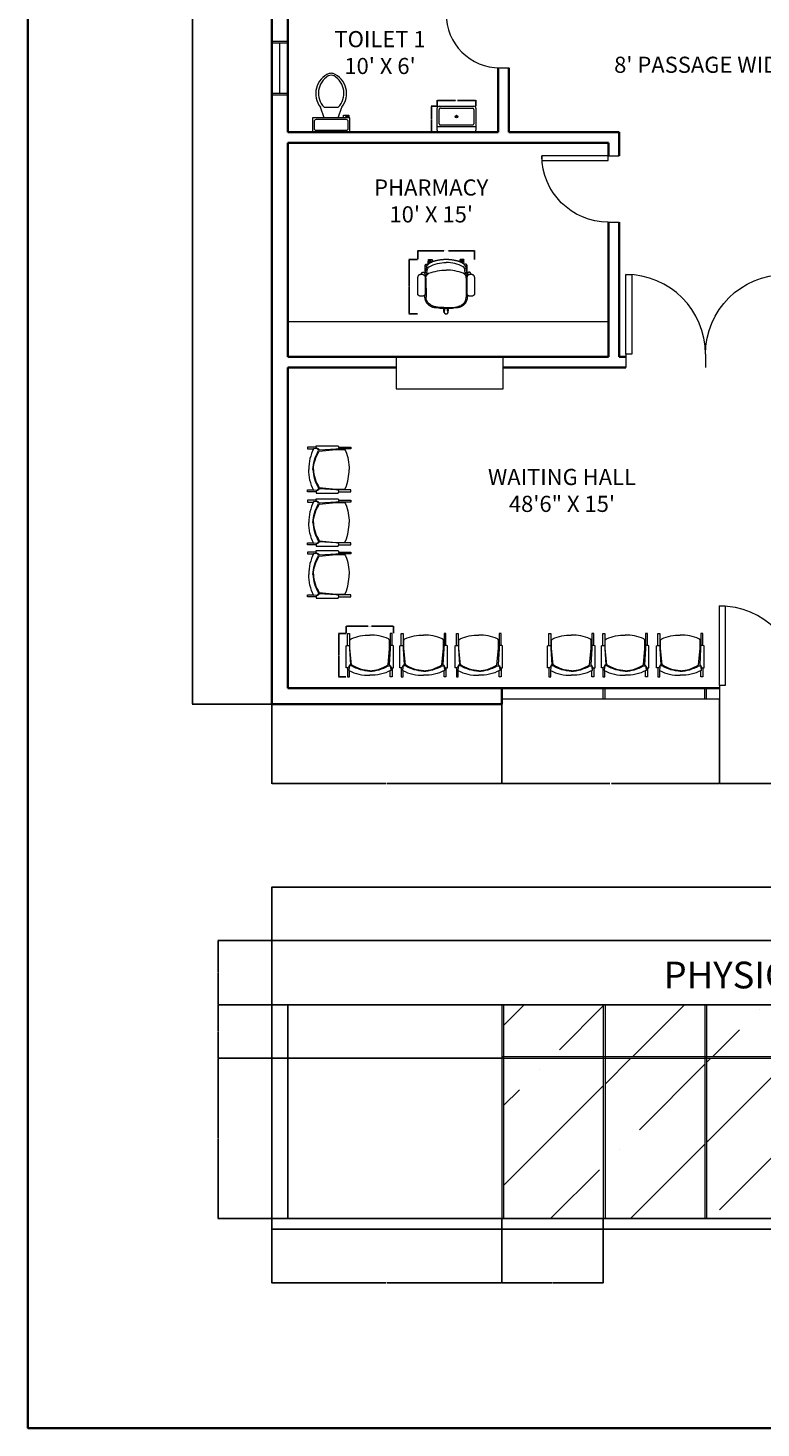
# Model space of a CAD drawing. Units: inches. Extents: x 7245 to 8143, y 15548 to 17244.
# Tile 1 of 5: x 7245 to 7657, y 15548 to 16334. Entities that reach past the tile are written whole.
import ezdxf

# ---------------------------------------------------------------- set-up
doc = ezdxf.new("R2010")
doc.units = ezdxf.units.IN
for name, color, linetype, lineweight in [('A-ANNO-DIMS', 2, 'Continuous', 18), ('A-ANNO-TEXT', 7, 'Continuous', 25), ('A-ANNO-TTLB', 7, 'Continuous', 35), ('A-AREA-IDEN', 7, 'Continuous', 18), ('A-DOOR', 3, 'Continuous', 18), ('A-ELEV', 7, 'Continuous', 25), ('A-ELEV-GLAZ', 4, 'Continuous', 18), ('A-ELEV-PATT', 252, 'Continuous', 13), ('A-FLOR-CASE', 9, 'Continuous', 20), ('A-FLOR-FIXT', 9, 'Continuous', 18), ('A-FURN', 8, 'Continuous', 18), ('A-GLAZ', 4, 'Continuous', 18), ('A-WALL', 7, 'Continuous', 35)]:
    doc.layers.add(name, color=color, linetype=linetype, lineweight=lineweight)
doc.styles.get("Standard").update_dxf_attribs({"font": 'arial.ttf'})
doc.dimstyles.get("Standard").update_dxf_attribs({"dimtxt": 0.18, "dimasz": 0.18, "dimexe": 0.18, "dimexo": 0.0625, "dimgap": 0.09, "dimtad": 0, "dimtih": 1, "dimtoh": 1, "dimdec": 4, "dimzin": 0, "dimdsep": 46, "dimtxsty": 'Standard', "dimcen": 0.09, "dimadec": 0, "dimazin": 0, "dimtfac": 1, "dimtdec": 4, "dimtofl": 0, "dimtmove": 0, "dimatfit": 3, "dimfxl": 1, "dimtolj": 1, "dimtzin": 0, "dimarcsym": 0})

# ---------------------------------------------------------------- blocks, each defined once
blk = doc.blocks.new('*U2')
for p, q in [((-600, 0), (-600, 100)), ((0, 0), (0, 100))]:
    blk.add_line(p, q)
blk.add_lwpolyline([(0, 0), (0, -600), (-43.75, -600), (-43.75, 0)], close=True)
blk.add_arc((0, 0), 600, 180, 270)
blk = doc.blocks.new('fdss')
at = {"color": 0}
for p, q in [((426, 240), (196, 239)), ((470, 236), (480, 226)), ((480, 225), (479, 223)), ((482, 204), (480, 210)), ((484, 228), (520, 224)), ((617, 196), (646, 196)), ((618, 179), (646, 179)), ((647, 195), (647, 179)), ((426, -240), (196, -239)), ((470, -236), (480, -226)), ((480, -225), (479, -223)), ((482, -204), (480, -210)), ((484, -228), (520, -224)), ((617, -196), (646, -196)), ((618, -179), (646, -179)), ((647, -195), (647, -179))]:
    blk.add_line(p, q, dxfattribs=at)
for points in [[(505, 245), (520, 247), (546, 249), (551, 249)], [(566, 236), (554, 235), (512, 240)], [(33, 21), (34, 20), (36, 19), (37, 18), (37, 18), (39, 18)], [(39, 18), (41, 17), (43, 17), (46, 16), (47, 16), (50, 16), (53, 16), (55, 16), (57, 16), (60, 16), (63, 16)], [(75, -28), (75, 0), (75, 28)], [(33, -21), (34, -20), (36, -19), (37, -18), (37, -18), (39, -18)], [(39, -18), (41, -17), (43, -17), (46, -16), (47, -16), (50, -16), (53, -16), (55, -16), (57, -16), (60, -16), (63, -16)], [(505, -245), (520, -247), (546, -249), (551, -249)], [(566, -236), (554, -235), (512, -240)]]:
    blk.add_lwpolyline(points, dxfattribs=at)
at = {"color": 0, "extrusion": (0, 0, -1)}
for centre, major_axis, start_param, end_param in [((445, 42), (-262, 262), 5.459154, 5.874691), ((201, 128), (-79, 79), 5.969012, 7.027382), ((424, 173), (47, 47), -0.751727, 0.301996), ((424, 175), (54.1, 54.1), -0.544214, -0.156468), ((514, 220), (24.9, 24.9), 3.662908, 4.015109), ((484, 224), (3.3, 3.3), 4.243712, 5.205719), ((484, 229), (-1.47, 1.47), 3.927418, 5.578652), ((-41, 3), (553, 91), -0.204201, 0.167634), ((500, 224), (-12.9, 12.9), 5.819354, 6.506047), ((509, 207), (26.9, 26.9), -1.329065, -0.883773), ((521, 177), (-33.1, 33.1), 0.763307, 1.830683), ((550, 228), (14.8, 14.8), -0.735707, 0.161366), ((545, 180), (-39.3, 39.3), 0.935679, 1.762262), ((193, 0), (-296, 296), 1.856147, 2.355859), ((566, 238), (1.31, 1.31), 0.929037, 2.293349), ((563, 238), (-2.9, 2.9), 1.793197, 2.458506), ((597, 186), (15.6, 15.6), -0.947253, 1.474381), ((621, 198), (-1.12, 1.12), 2.396655, 3.926991), ((621, 177), (-1.12, 1.12), 0.785398, 2.315734), ((646, 195), (0.539, 0.539), -0.785398, 0.785398), ((646, 179), (-0.539, 0.539), 2.356195, 3.926991)]:
    blk.add_ellipse(centre, major_axis=major_axis, ratio=1, start_param=start_param, end_param=end_param, dxfattribs=at)
at = {"color": 0}
for centre, major_axis, start_param, end_param in [((445, -42), (262, 262), 2.317561, 2.733098), ((-41, -3), (-553, 91), 2.937392, 3.309227), ((193, 0), (296, 296), 4.99774, 5.497452), ((201, -128), (79, 79), 2.82742, 3.885789), ((424, -173), (-47, 47), 2.389866, 3.443588), ((424, -175), (-54.1, 54.1), 2.597378, 2.985125), ((514, -220), (-24.9, 24.9), 0.521315, 0.873517), ((484, -224), (-3.3, 3.3), 1.102119, 2.064126), ((484, -229), (1.47, 1.47), 0.785825, 2.437059), ((500, -224), (12.9, 12.9), 2.677762, 3.364454), ((509, -207), (-26.9, 26.9), 1.812527, 2.25782), ((521, -177), (33.1, 33.1), 3.9049, 4.972275), ((550, -228), (-14.8, 14.8), 2.405886, 3.302959), ((545, -180), (39.3, 39.3), 4.077272, 4.903855), ((566, -238), (-1.31, 1.31), 4.07063, 5.434941), ((563, -238), (2.9, 2.9), 4.93479, 5.600098), ((597, -186), (15.6, 15.6), 3.765136, 6.18677), ((621, -177), (1.12, 1.12), 3.926991, 5.457327), ((621, -198), (1.12, 1.12), 5.538248, 7.068583), ((646, -179), (0.539, 0.539), 5.497787, 7.068583), ((646, -195), (-0.539, 0.539), 2.356195, 3.926991)]:
    blk.add_ellipse(centre, major_axis=major_axis, ratio=1, start_param=start_param, end_param=end_param, dxfattribs=at)
for points, weights, knots in [([(436, 337), (338, 337), (240, 337), (234, 338), (228, 335), (217, 328), (212, 315), (204, 293), (212, 271), (217, 258), (228, 251), (234, 248), (240, 248)], [1, 1, 1, 0.962754439438, 1, 0.939418827348, 1, 0.934055427035, 1, 0.939418827348, 1, 0.962754439438, 1], [0, 0, 0, 1, 1, 1.54757, 1.54757, 2.247301, 2.247301, 2.977684, 2.977684, 3.677415, 3.677415, 4.224984, 4.224984, 4.224984]), ([(436, 337), (443, 338), (449, 335), (460, 328), (464, 315), (473, 293), (464, 271), (460, 258), (449, 251), (443, 248), (436, 248), (338, 248), (240, 248)], [1, 0.96275443944, 1, 0.939418827348, 1, 0.934055427035, 1, 0.939418827348, 1, 0.96275443944, 1, 1, 1], [0, 0, 0, 0.54757, 0.54757, 1.247301, 1.247301, 1.977684, 1.977684, 2.677415, 2.677415, 3.224984, 3.224984, 4.224984, 4.224984, 4.224984]), ([(227, 252), (219, 252), (211, 252), (156, 255), (115, 218), (74, 180), (72, 125), (63, 75), (63, 25), (63, 13), (62, 0), (63, -13), (63, -25), (63, -75), (72, -125), (74, -180), (115, -218), (156, -255), (211, -252), (219, -252), (227, -252)], [1, 1, 1, 0.920970329426, 1, 0.920970329426, 1, 0.996764637726, 1, 1, 1, 1, 1, 0.996764637726, 1, 0.920970329426, 1, 0.920970329426, 1, 1, 1], [0, 0, 0, 1, 1, 1.800466, 1.800466, 2.600931, 2.600931, 2.761856, 2.761856, 3.761856, 3.761856, 4.761856, 4.761856, 4.922781, 4.922781, 5.723247, 5.723247, 6.523712, 6.523712, 7.523712, 7.523712, 7.523712]), ([(447, 248), (506, 249), (566, 251), (577, 251), (585, 244), (591, 239), (592, 232), (592, 228), (590, 225), (589, 221), (585, 219)], [1, 1, 1, 0.935512434708, 1, 0.918468104225, 1, 0.965843473499, 1, 0.972653000165, 1], [0, 0, 0, 1, 1, 1.722179, 1.722179, 2.535393, 2.535393, 3.059628, 3.059628, 3.528435, 3.528435, 3.528435]), ([(468, 296), (480, 296), (489, 288), (493, 285), (494, 280), (496, 274), (494, 268), (488, 255), (474, 254), (463, 254), (452, 253)], [1, 0.943338632687, 1, 0.968267368414, 1, 0.9394851057, 1, 0.864198855487, 1, 1, 1], [0, 0, 0, 0.676489, 0.676489, 1.181677, 1.181677, 1.881021, 1.881021, 2.935502, 2.935502, 3.935502, 3.935502, 3.935502]), ([(591, 211), (619, 173), (629, 128), (645, 65), (645, 0), (645, -65), (629, -128), (619, -173), (591, -211)], [1, 0.979760898136, 1, 0.992391068779, 1, 0.992391068779, 1, 0.979760898136, 1], [0, 0, 0, 0.403066, 0.403066, 0.649944, 0.649944, 0.896822, 0.896822, 1.299888, 1.299888, 1.299888]), ([(592, 211), (618, 216), (643, 209), (646, 209), (646, 206), (646, 203), (646, 199), (646, 198), (644, 198), (630, 198), (616, 198)], [1, 0.974666881773, 1, 0.783317345499, 1, 1, 1, 0.707106807826, 1, 1, 1], [0, 0, 0, 0.451139, 0.451139, 1.792762, 1.792762, 2.792762, 2.792762, 4.363559, 4.363559, 5.363559, 5.363559, 5.363559]), ([(618, 177), (631, 177), (644, 177), (645, 177), (645, 176), (646, 176), (646, 175), (646, 172), (646, 168), (646, 166), (643, 165), (631, 161), (619, 161)], [1, 1, 1, 0.923879528314, 1, 0.923879528314, 1, 1, 1, 0.783317456604, 1, 0.992237440768, 1], [0, 0, 0, 1, 1, 1.785398, 1.785398, 2.570796, 2.570796, 3.570796, 3.570796, 4.912419, 4.912419, 5.161781, 5.161781, 5.161781]), ([(33, -20), (22, -27), (10, -20), (-1, -13), (0, 0), (-1, 13), (10, 20), (22, 27), (33, 20)], [1, 0.85579821339, 1, 0.85579821339, 1, 0.855798213391, 1, 0.855798213391, 1], [0, 0, 0, 1.087409, 1.087409, 2.174818, 2.174818, 3.262227, 3.262227, 4.349636, 4.349636, 4.349636]), ([(12, 21), (13, 23), (15, 23), (39, 29), (63, 25)], [1, 0.873023611703, 1, 0.980536821249, 1], [0, 0, 0, 1.018856, 1.018856, 1.414094, 1.414094, 1.414094]), ([(12, -21), (13, -23), (15, -23), (39, -29), (63, -25)], [1, 0.873023611717, 1, 0.980536821249, 1], [0, 0, 0, 1.018856, 1.018856, 1.414094, 1.414094, 1.414094]), ([(618, -177), (631, -177), (644, -177), (645, -177), (645, -176), (646, -176), (646, -175), (646, -172), (646, -168), (646, -166), (643, -165), (631, -161), (619, -161)], [1, 1, 1, 0.923879528318, 1, 0.923879528318, 1, 1, 1, 0.783317456602, 1, 0.992237440768, 1], [0, 0, 0, 1, 1, 1.785398, 1.785398, 2.570796, 2.570796, 3.570796, 3.570796, 4.912419, 4.912419, 5.161781, 5.161781, 5.161781]), ([(464, -271), (460, -258), (449, -251), (443, -248), (436, -248), (338, -248), (240, -248), (234, -248), (228, -251), (217, -258), (212, -271), (204, -293), (212, -315), (217, -328), (228, -335), (234, -338), (240, -337), (338, -337), (436, -337)], [1, 0.939418827349, 1, 0.96275443944, 1, 1, 1, 0.962754439438, 1, 0.939418827349, 1, 0.934055427035, 1, 0.939418827348, 1, 0.962754439438, 1, 1, 1], [0, 0, 0, 0.699731, 0.699731, 1.247301, 1.247301, 2.247301, 2.247301, 2.794871, 2.794871, 3.494602, 3.494602, 4.224984, 4.224984, 4.924715, 4.924715, 5.472285, 5.472285, 6.472285, 6.472285, 6.472285]), ([(464, -271), (473, -293), (464, -315), (460, -328), (449, -335), (443, -338), (436, -337)], [1, 0.934055427035, 1, 0.939418827348, 1, 0.96275443944, 1], [0, 0, 0, 0.730383, 0.730383, 1.430114, 1.430114, 1.977684, 1.977684, 1.977684]), ([(447, -248), (506, -249), (566, -251), (577, -251), (585, -244), (591, -239), (592, -232), (592, -228), (590, -225), (589, -221), (585, -219)], [1, 1, 1, 0.935512434708, 1, 0.918468104224, 1, 0.965843473499, 1, 0.972653000166, 1], [0, 0, 0, 1, 1, 1.722179, 1.722179, 2.535393, 2.535393, 3.059628, 3.059628, 3.528435, 3.528435, 3.528435]), ([(468, -296), (480, -296), (489, -288), (493, -285), (494, -280), (496, -274), (494, -268), (488, -255), (474, -254), (463, -254), (452, -253)], [1, 0.943338632687, 1, 0.968267368413, 1, 0.9394851057, 1, 0.864198855486, 1, 1, 1], [0, 0, 0, 0.676489, 0.676489, 1.181677, 1.181677, 1.881021, 1.881021, 2.935502, 2.935502, 3.935502, 3.935502, 3.935502]), ([(592, -211), (618, -216), (643, -209), (646, -209), (646, -206), (646, -203), (646, -199), (646, -198), (644, -198), (630, -198), (616, -198)], [1, 0.974666881774, 1, 0.7833173455, 1, 1, 1, 0.707106807832, 1, 1, 1], [0, 0, 0, 0.451139, 0.451139, 1.792762, 1.792762, 2.792762, 2.792762, 4.363559, 4.363559, 5.363559, 5.363559, 5.363559])]:
    blk.add_rational_spline(points, weights, degree=2, knots=knots, dxfattribs=at)
blk = doc.blocks.new('chair033')
at = {"color": 0, "lineweight": -2}
for points in [[(-230, -108), (-230, 17), (-210, 17), (-210, -113)], [(230, -108), (230, 17), (210, 17), (210, -113)], [(-230, -338), (-230, -428), (-210, -428), (-210, -366)], [(230, -338), (230, -428), (210, -428), (210, -366)]]:
    blk.add_lwpolyline(points, dxfattribs=at)
for points in [[(1, -367, -0.129806), (-187, -307), (-204, -137), (-204, -56, -0.30894), (-191, -37, -0.09648), (0, 0, -0.09648)], [(-1, -367, 0.129806), (187, -307), (204, -137), (204, -56, 0.30894), (191, -37, 0.09648), (0, 0, 0.09648)], [(1, -372, -0.119401), (-187, -317, 0.398658), (-212, -327), (-215, -363, 0.13244), (0, -413)], [(-1, -372, 0.119401), (187, -317, -0.398658), (212, -327), (215, -363, -0.13244), (0, -413)]]:
    blk.add_lwpolyline(points, format="xyb", dxfattribs=at)
for points in [[(-244, -337), (-244, -157), (-244, -112, -0.285714), (-209, -112), (-209, -137), (-199, -306, 0.220172), (-212, -317), (-222, -337)], [(244, -337), (244, -157), (244, -112, 0.285714), (209, -112), (209, -137), (199, -306, -0.220172), (212, -317), (222, -337)]]:
    blk.add_lwpolyline(points, format="xyb", close=True, dxfattribs=at)
blk = doc.blocks.new('*U9')
for p, q in [((0, 0), (0, 100)), ((600, 0), (600, 100))]:
    blk.add_line(p, q)
blk.add_lwpolyline([(0, 0), (0, -600), (43.75, -600), (43.75, 0)], close=True)
blk.add_arc((0, 0), 600, 270, 0)
blk = doc.blocks.new('Toilet - top')
for p, q in [((9.5, -6), (9.5, -2)), ((-10, -8.5), (-8, -8.5)), ((-10, -9.5), (-10, -8.5)), ((-7, -9.5), (-10, -9.5)), ((-8, -8.5), (-8, -8)), ((-7, -8), (-7, -9.5)), ((-4, -8), (-6, -14)), ((4, -14), (-4, -14)), ((4, -8), (6, -14))]:
    blk.add_line(p, q)
blk.add_lwpolyline([(10.5, -8), (10.5, 0), (-10.5, 0), (-10.5, -8)], close=True)
for points in [[(-9.5, -2), (-9.5, -6)], [(8.5, -1), (-8.5, -1)], [(-8.5, -7), (8.5, -7)]]:
    blk.add_lwpolyline(points)
for centre, radius, start, end in [((-8.62, -1.88), 0.884, 81.8699, 188.1301), ((-8.62, -6.12), 0.884, 171.8699, 278.1301), ((8.62, -1.88), 0.884, 351.8699, 98.1301), ((8.62, -6.12), 0.884, 261.8699, 8.1301), ((3.52, -21.58), 12.17, 141.46911, 247.97143), ((4.2, -21.82), 11.33, 136.36773, 238.94682), ((-3.52, -21.58), 12.17, 292.02843, 38.53071), ((-4.2, -21.82), 11.33, 301.05301, 43.63209), ((0, -27.88), 4, 245.73182, 294.26817), ((0, -29), 4, 254.86053, 285.13947)]:
    blk.add_arc(centre, radius, start, end)
blk = doc.blocks.new('Sink-single - 30 in top')
blk.add_line((-15, -3.999996), (15, -3.999996))
for points in [[(-13.5, 0), (13.5, 0)], [(-15, -18.499996), (-15, -1.5)], [(-13.5, -17.499996), (-13.5, -6.499996)], [(-12.5, -5.499996), (12.5, -5.499996)], [(13.5, -6.499996), (13.5, -17.499996)], [(15, -1.5), (15, -18.499996)], [(13.5, -19.999996), (-13.5, -19.999996)], [(12.5, -18.499996), (-12.5, -18.499996)]]:
    blk.add_lwpolyline(points)
for radius in [1, 0.5]:
    blk.add_circle((0, -11.999996), radius)
for centre, radius, start, end in [((-13.5, -1.5), 1.5, 90, 180), ((-12.5, -6.499996), 1, 90, 180), ((12.5, -6.499996), 1, 0, 90), ((13.5, -1.5), 1.5, 0, 90), ((-13.5, -18.499996), 1.5, 180, 270), ((-12.5, -17.499996), 1, 180, 270), ((12.5, -17.499996), 1, 270, 0), ((13.5, -18.499996), 1.5, 270, 0)]:
    blk.add_arc(centre, radius, start, end)
blk = doc.blocks.new('WINDOW-30IN-PLAN')
for p, q in [((30, 9), (0, 9)), ((0, 9), (0, 0)), ((1, 9), (1, 0)), ((29, 0), (29, 9)), ((30, 0), (30, 9)), ((29, 4.5), (1, 4.5)), ((0, 0), (30, 0))]:
    blk.add_line(p, q)
blk = doc.blocks.new('*D18')
at = {"layer": 'A-ANNO-DIMS', "color": 0, "lineweight": -2, "transparency": 16777216}
for p, q in [((7423.74, 15993.99), (7423.74, 15998.1)), ((7423.92, 15997.92), (7436.12, 15997.92)), ((7450.22, 15997.92), (7438.02, 15997.92)), ((7450.4, 15993.99), (7450.4, 15998.1))]:
    blk.add_line(p, q, dxfattribs=at)
at = {"layer": 'A-ANNO-DIMS', "color": 0, "transparency": 16777216}
for points in [[(7423.92, 15997.95), (7423.92, 15997.89), (7423.74, 15997.92)], [(7450.22, 15997.95), (7450.22, 15997.89), (7450.4, 15997.92)]]:
    blk.add_solid(points, dxfattribs=at)
at = {"layer": 'Defpoints', "color": 0, "transparency": 16777216}
for p in [(7423.74, 15993.93), (7450.4, 15997.92), (7450.4, 15993.93)]:
    blk.add_point(p, dxfattribs=at)
at = {"layer": 'A-ANNO-DIMS', "color": 0, "transparency": 16777216, "insert": (7437.07, 15997.92), "char_height": 0.18, "attachment_point": 5}
blk.add_mtext('\\A1;CHAIR 27 TYP.', dxfattribs=at)
blk = doc.blocks.new('*D19')
at = {"layer": 'A-ANNO-DIMS', "color": 0, "lineweight": -2, "transparency": 16777216}
for p, q in [((7423.68, 15993.93), (7419.56, 15993.93)), ((7419.74, 15993.75), (7419.74, 15981.95)), ((7419.74, 15969.79), (7419.74, 15981.59)), ((7423.68, 15969.61), (7419.56, 15969.61))]:
    blk.add_line(p, q, dxfattribs=at)
at = {"layer": 'A-ANNO-DIMS', "color": 0, "transparency": 16777216}
for points in [[(7419.71, 15993.75), (7419.77, 15993.75), (7419.74, 15993.93)], [(7419.71, 15969.79), (7419.77, 15969.79), (7419.74, 15969.61)]]:
    blk.add_solid(points, dxfattribs=at)
at = {"layer": 'Defpoints', "color": 0, "transparency": 16777216}
for p in [(7419.74, 15993.93), (7423.74, 15993.93), (7423.74, 15969.61)]:
    blk.add_point(p, dxfattribs=at)
at = {"layer": 'A-ANNO-DIMS', "color": 0, "transparency": 16777216, "insert": (7419.74, 15981.77), "char_height": 0.18, "attachment_point": 5}
blk.add_mtext('\\A1;24 TYP.', dxfattribs=at)
blk = doc.blocks.new('*D24')
at = {"layer": 'A-ANNO-DIMS', "color": 0, "lineweight": -2, "transparency": 16777216}
for p, q in [((7474.87, 16289.75), (7474.87, 16293.13)), ((7475.05, 16292.95), (7485.12, 16292.95)), ((7496.43, 16292.95), (7486.37, 16292.95)), ((7496.61, 16289.75), (7496.61, 16293.13))]:
    blk.add_line(p, q, dxfattribs=at)
at = {"layer": 'A-ANNO-DIMS', "color": 0, "transparency": 16777216}
for points in [[(7475.05, 16292.98), (7475.05, 16292.92), (7474.87, 16292.95)], [(7496.43, 16292.98), (7496.43, 16292.92), (7496.61, 16292.95)]]:
    blk.add_solid(points, dxfattribs=at)
at = {"layer": 'Defpoints', "color": 0, "transparency": 16777216}
for p in [(7474.87, 16292.95), (7474.87, 16289.69), (7496.61, 16289.69)]:
    blk.add_point(p, dxfattribs=at)
at = {"layer": 'A-ANNO-DIMS', "color": 0, "transparency": 16777216, "insert": (7485.74, 16292.95), "char_height": 0.18, "attachment_point": 5}
blk.add_mtext('\\A1;BASIN 22', dxfattribs=at)
blk = doc.blocks.new('*D25')
at = {"layer": 'A-ANNO-DIMS', "color": 0, "lineweight": -2, "transparency": 16777216}
for p, q in [((7474.81, 16289.69), (7471.43, 16289.69)), ((7471.61, 16289.51), (7471.61, 16282.62)), ((7474.81, 16275.19), (7471.43, 16275.19)), ((7471.61, 16275.37), (7471.61, 16282.26))]:
    blk.add_line(p, q, dxfattribs=at)
at = {"layer": 'A-ANNO-DIMS', "color": 0, "transparency": 16777216}
for points in [[(7471.58, 16289.51), (7471.64, 16289.51), (7471.61, 16289.69)], [(7471.58, 16275.37), (7471.64, 16275.37), (7471.61, 16275.19)]]:
    blk.add_solid(points, dxfattribs=at)
at = {"layer": 'Defpoints', "color": 0, "transparency": 16777216}
for p in [(7474.87, 16289.69), (7471.61, 16275.19), (7474.87, 16275.19)]:
    blk.add_point(p, dxfattribs=at)
at = {"layer": 'A-ANNO-DIMS', "color": 0, "transparency": 16777216, "insert": (7471.61, 16282.44), "char_height": 0.18, "attachment_point": 5}
blk.add_mtext('\\A1;14', dxfattribs=at)
blk = doc.blocks.new('*D26')
at = {"layer": 'A-ANNO-DIMS', "color": 0, "lineweight": -2, "transparency": 16777216}
for p, q in [((7463.99, 16203.82), (7463.99, 16208.71)), ((7464.17, 16208.53), (7478.58, 16208.53)), ((7495.64, 16208.53), (7481.23, 16208.53)), ((7495.82, 16203.81), (7495.82, 16208.71))]:
    blk.add_line(p, q, dxfattribs=at)
at = {"layer": 'A-ANNO-DIMS', "color": 0, "transparency": 16777216}
for points in [[(7464.17, 16208.56), (7464.17, 16208.5), (7463.99, 16208.53)], [(7495.64, 16208.56), (7495.64, 16208.5), (7495.82, 16208.53)]]:
    blk.add_solid(points, dxfattribs=at)
at = {"layer": 'Defpoints', "color": 0, "transparency": 16777216}
for p in [(7495.82, 16208.53), (7463.99, 16203.75), (7495.82, 16203.75)]:
    blk.add_point(p, dxfattribs=at)
at = {"layer": 'A-ANNO-DIMS', "color": 0, "transparency": 16777216, "insert": (7479.91, 16208.53), "char_height": 0.18, "attachment_point": 5}
blk.add_mtext('\\A1;DESK CHAIR 32 TYP.', dxfattribs=at)
blk = doc.blocks.new('*D27')
at = {"layer": 'A-ANNO-DIMS', "color": 0, "lineweight": -2, "transparency": 16777216}
for p, q in [((7463.93, 16203.75), (7459.03, 16203.75)), ((7459.21, 16203.57), (7459.21, 16188.68)), ((7459.21, 16173.42), (7459.21, 16188.31)), ((7463.92, 16173.24), (7459.03, 16173.24))]:
    blk.add_line(p, q, dxfattribs=at)
at = {"layer": 'A-ANNO-DIMS', "color": 0, "transparency": 16777216}
for points in [[(7459.18, 16203.57), (7459.24, 16203.57), (7459.21, 16203.75)], [(7459.18, 16173.42), (7459.24, 16173.42), (7459.21, 16173.24)]]:
    blk.add_solid(points, dxfattribs=at)
at = {"layer": 'Defpoints', "color": 0, "transparency": 16777216}
for p in [(7459.21, 16203.75), (7463.99, 16203.75), (7463.99, 16173.24)]:
    blk.add_point(p, dxfattribs=at)
at = {"layer": 'A-ANNO-DIMS', "color": 0, "transparency": 16777216, "insert": (7459.21, 16188.5), "char_height": 0.18, "attachment_point": 5}
blk.add_mtext('\\A1;31 TYP.', dxfattribs=at)
blk = doc.blocks.new('*D43')
at = {"layer": 'A-ANNO-DIMS', "color": 0, "lineweight": -2, "transparency": 16777216}
for p, q in [((7382.02, 16842.19), (7337.4, 16842.19)), ((7337.58, 16842.01), (7337.58, 16398.37)), ((7337.58, 15954.37), (7337.58, 16398.01)), ((7382.02, 15954.19), (7337.4, 15954.19))]:
    blk.add_line(p, q, dxfattribs=at)
at = {"layer": 'A-ANNO-DIMS', "color": 0, "transparency": 16777216}
for points in [[(7337.55, 16842.01), (7337.61, 16842.01), (7337.58, 16842.19)], [(7337.55, 15954.37), (7337.61, 15954.37), (7337.58, 15954.19)]]:
    blk.add_solid(points, dxfattribs=at)
at = {"layer": 'Defpoints', "color": 0, "transparency": 16777216}
for p in [(7337.58, 16842.19), (7382.08, 16842.19), (7382.08, 15954.19)]:
    blk.add_point(p, dxfattribs=at)
at = {"layer": 'A-ANNO-DIMS', "color": 0, "transparency": 16777216, "insert": (7337.58, 16398.19), "char_height": 0.18, "attachment_point": 5}
blk.add_mtext('\\A1;888', dxfattribs=at)
blk = doc.blocks.new('*D44')
at = {"layer": 'A-ANNO-DIMS', "color": 0, "lineweight": -2, "transparency": 16777216}
for p, q in [((7382.08, 15954.13), (7382.08, 15909.51)), ((7511.08, 15954.13), (7511.08, 15909.51)), ((7382.26, 15909.69), (7446.3, 15909.69)), ((7510.9, 15909.69), (7446.86, 15909.69))]:
    blk.add_line(p, q, dxfattribs=at)
at = {"layer": 'A-ANNO-DIMS', "color": 0, "transparency": 16777216}
for points in [[(7382.26, 15909.72), (7382.26, 15909.66), (7382.08, 15909.69)], [(7510.9, 15909.72), (7510.9, 15909.66), (7511.08, 15909.69)]]:
    blk.add_solid(points, dxfattribs=at)
at = {"layer": 'Defpoints', "color": 0, "transparency": 16777216}
for p in [(7382.08, 15954.19), (7511.08, 15954.19), (7511.08, 15909.69)]:
    blk.add_point(p, dxfattribs=at)
at = {"layer": 'A-ANNO-DIMS', "color": 0, "transparency": 16777216, "insert": (7446.58, 15909.69), "char_height": 0.18, "attachment_point": 5}
blk.add_mtext('\\A1;129', dxfattribs=at)
blk = doc.blocks.new('*D45')
at = {"layer": 'A-ANNO-DIMS', "color": 0, "lineweight": -2, "transparency": 16777216}
for p, q in [((7511.08, 15957.13), (7511.08, 15909.51)), ((7633.26, 15957.13), (7633.26, 15909.51)), ((7511.26, 15909.69), (7571.72, 15909.69)), ((7633.08, 15909.69), (7572.63, 15909.69))]:
    blk.add_line(p, q, dxfattribs=at)
at = {"layer": 'A-ANNO-DIMS', "color": 0, "transparency": 16777216}
for points in [[(7511.26, 15909.72), (7511.26, 15909.66), (7511.08, 15909.69)], [(7633.08, 15909.72), (7633.08, 15909.66), (7633.26, 15909.69)]]:
    blk.add_solid(points, dxfattribs=at)
at = {"layer": 'Defpoints', "color": 0, "transparency": 16777216}
for p in [(7511.08, 15957.19), (7633.26, 15957.19), (7633.26, 15909.69)]:
    blk.add_point(p, dxfattribs=at)
at = {"layer": 'A-ANNO-DIMS', "color": 0, "transparency": 16777216, "insert": (7572.17, 15909.69), "char_height": 0.18, "attachment_point": 5}
blk.add_mtext('\\A1;122.18', dxfattribs=at)
blk = doc.blocks.new('*D46')
at = {"layer": 'A-ANNO-DIMS', "color": 0, "lineweight": -2, "transparency": 16777216}
for p, q in [((7633.26, 15957.13), (7633.26, 15909.51)), ((7722.64, 15957.13), (7722.64, 15909.51)), ((7633.44, 15909.69), (7677.55, 15909.69)), ((7722.46, 15909.69), (7678.34, 15909.69))]:
    blk.add_line(p, q, dxfattribs=at)
at = {"layer": 'A-ANNO-DIMS', "color": 0, "transparency": 16777216}
for points in [[(7633.44, 15909.72), (7633.44, 15909.66), (7633.26, 15909.69)], [(7722.46, 15909.72), (7722.46, 15909.66), (7722.64, 15909.69)]]:
    blk.add_solid(points, dxfattribs=at)
at = {"layer": 'Defpoints', "color": 0, "transparency": 16777216}
for p in [(7633.26, 15957.19), (7722.64, 15957.19), (7722.64, 15909.69)]:
    blk.add_point(p, dxfattribs=at)
at = {"layer": 'A-ANNO-DIMS', "color": 0, "transparency": 16777216, "insert": (7677.95, 15909.69), "char_height": 0.18, "attachment_point": 5}
blk.add_mtext('\\A1;89.37', dxfattribs=at)
blk = doc.blocks.new('*D69')
at = {"layer": 'A-ANNO-DIMS', "color": 0, "lineweight": -2, "transparency": 16777216}
for p, q in [((7382.08, 15821.68), (7382.08, 15851.81)), ((7382.26, 15851.63), (7681.79, 15851.63)), ((7981.9, 15851.63), (7682.37, 15851.63)), ((7982.08, 15821.68), (7982.08, 15851.81))]:
    blk.add_line(p, q, dxfattribs=at)
at = {"layer": 'A-ANNO-DIMS', "color": 0, "transparency": 16777216}
for points in [[(7382.26, 15851.66), (7382.26, 15851.6), (7382.08, 15851.63)], [(7981.9, 15851.66), (7981.9, 15851.6), (7982.08, 15851.63)]]:
    blk.add_solid(points, dxfattribs=at)
at = {"layer": 'Defpoints', "color": 0, "transparency": 16777216}
for p in [(7982.08, 15851.63), (7382.08, 15821.62), (7982.08, 15821.62)]:
    blk.add_point(p, dxfattribs=at)
at = {"layer": 'A-ANNO-DIMS', "color": 0, "transparency": 16777216, "insert": (7682.08, 15851.63), "char_height": 0.18, "attachment_point": 5}
blk.add_mtext('\\A1;600', dxfattribs=at)
blk = doc.blocks.new('*D71')
at = {"layer": 'A-ANNO-DIMS', "color": 0, "lineweight": -2, "transparency": 16777216}
for p, q in [((7382.08, 15665.56), (7382.08, 15629.42)), ((7511.08, 15665.56), (7511.08, 15629.42)), ((7382.26, 15629.6), (7446.3, 15629.6)), ((7510.9, 15629.6), (7446.86, 15629.6))]:
    blk.add_line(p, q, dxfattribs=at)
at = {"layer": 'A-ANNO-DIMS', "color": 0, "transparency": 16777216}
for points in [[(7382.26, 15629.63), (7382.26, 15629.57), (7382.08, 15629.6)], [(7510.9, 15629.63), (7510.9, 15629.57), (7511.08, 15629.6)]]:
    blk.add_solid(points, dxfattribs=at)
at = {"layer": 'Defpoints', "color": 0, "transparency": 16777216}
for p in [(7382.08, 15665.62), (7511.08, 15665.62), (7511.08, 15629.6)]:
    blk.add_point(p, dxfattribs=at)
at = {"layer": 'A-ANNO-DIMS', "color": 0, "transparency": 16777216, "insert": (7446.58, 15629.6), "char_height": 0.18, "attachment_point": 5}
blk.add_mtext('\\A1;129', dxfattribs=at)
blk = doc.blocks.new('*D72')
at = {"layer": 'A-ANNO-DIMS', "color": 0, "lineweight": -2, "transparency": 16777216}
for p, q in [((7511.08, 15665.56), (7511.08, 15629.42)), ((7568.08, 15665.56), (7568.08, 15629.42)), ((7511.26, 15629.6), (7539.36, 15629.6)), ((7567.9, 15629.6), (7539.8, 15629.6))]:
    blk.add_line(p, q, dxfattribs=at)
at = {"layer": 'A-ANNO-DIMS', "color": 0, "transparency": 16777216}
for points in [[(7511.26, 15629.63), (7511.26, 15629.57), (7511.08, 15629.6)], [(7567.9, 15629.63), (7567.9, 15629.57), (7568.08, 15629.6)]]:
    blk.add_solid(points, dxfattribs=at)
at = {"layer": 'Defpoints', "color": 0, "transparency": 16777216}
for p in [(7511.08, 15665.62), (7568.08, 15665.62), (7568.08, 15629.6)]:
    blk.add_point(p, dxfattribs=at)
at = {"layer": 'A-ANNO-DIMS', "color": 0, "transparency": 16777216, "insert": (7539.58, 15629.6), "char_height": 0.18, "attachment_point": 5}
blk.add_mtext('\\A1;57', dxfattribs=at)
blk = doc.blocks.new('*D74')
at = {"layer": 'A-ANNO-DIMS', "color": 0, "lineweight": -2, "transparency": 16777216}
for p, q in [((7511.02, 15755.62), (7351.89, 15755.62)), ((7352.07, 15755.44), (7352.07, 15710.8)), ((7352.07, 15665.8), (7352.07, 15710.44)), ((7511.02, 15665.62), (7351.89, 15665.62))]:
    blk.add_line(p, q, dxfattribs=at)
at = {"layer": 'A-ANNO-DIMS', "color": 0, "transparency": 16777216}
for points in [[(7352.04, 15755.44), (7352.1, 15755.44), (7352.07, 15755.62)], [(7352.04, 15665.8), (7352.1, 15665.8), (7352.07, 15665.62)]]:
    blk.add_solid(points, dxfattribs=at)
at = {"layer": 'Defpoints', "color": 0, "transparency": 16777216}
for p in [(7352.07, 15755.62), (7511.08, 15755.62), (7511.08, 15665.62)]:
    blk.add_point(p, dxfattribs=at)
at = {"layer": 'A-ANNO-DIMS', "color": 0, "transparency": 16777216, "insert": (7352.07, 15710.62), "char_height": 0.18, "attachment_point": 5}
blk.add_mtext('\\A1;90', dxfattribs=at)
blk = doc.blocks.new('*D75')
at = {"layer": 'A-ANNO-DIMS', "color": 0, "lineweight": -2, "transparency": 16777216}
for p, q in [((7511.02, 15785.62), (7351.89, 15785.62)), ((7352.07, 15785.44), (7352.07, 15770.8)), ((7352.07, 15755.8), (7352.07, 15770.44)), ((7511.02, 15755.62), (7351.89, 15755.62))]:
    blk.add_line(p, q, dxfattribs=at)
at = {"layer": 'A-ANNO-DIMS', "color": 0, "transparency": 16777216}
for points in [[(7352.04, 15785.44), (7352.1, 15785.44), (7352.07, 15785.62)], [(7352.04, 15755.8), (7352.1, 15755.8), (7352.07, 15755.62)]]:
    blk.add_solid(points, dxfattribs=at)
at = {"layer": 'Defpoints', "color": 0, "transparency": 16777216}
for p in [(7352.07, 15785.62), (7511.08, 15785.62), (7511.08, 15755.62)]:
    blk.add_point(p, dxfattribs=at)
at = {"layer": 'A-ANNO-DIMS', "color": 0, "transparency": 16777216, "insert": (7352.07, 15770.62), "char_height": 0.18, "attachment_point": 5}
blk.add_mtext('\\A1;30', dxfattribs=at)
blk = doc.blocks.new('*D76')
at = {"layer": 'A-ANNO-DIMS', "color": 0, "lineweight": -2, "transparency": 16777216}
for p, q in [((7382.02, 15821.62), (7351.89, 15821.62)), ((7352.07, 15821.44), (7352.07, 15803.8)), ((7352.07, 15785.8), (7352.07, 15803.44)), ((7382.02, 15785.62), (7351.89, 15785.62))]:
    blk.add_line(p, q, dxfattribs=at)
at = {"layer": 'A-ANNO-DIMS', "color": 0, "transparency": 16777216}
for points in [[(7352.04, 15821.44), (7352.1, 15821.44), (7352.07, 15821.62)], [(7352.04, 15785.8), (7352.1, 15785.8), (7352.07, 15785.62)]]:
    blk.add_solid(points, dxfattribs=at)
at = {"layer": 'Defpoints', "color": 0, "transparency": 16777216}
for p in [(7352.07, 15821.62), (7382.08, 15821.62), (7382.08, 15785.62)]:
    blk.add_point(p, dxfattribs=at)
at = {"layer": 'A-ANNO-DIMS', "color": 0, "transparency": 16777216, "insert": (7352.07, 15803.62), "char_height": 0.18, "attachment_point": 5}
blk.add_mtext('\\A1;36', dxfattribs=at)

msp = doc.modelspace()

# ---------------------------------------------------------------- hatches: boundary and pattern name
at = {"layer": 'A-ELEV-PATT'}
h = msp.add_hatch(dxfattribs=at)
h.set_pattern_fill('ANSI35', color=256, scale=10)
h.paths.add_polyline_path([(7568.0838, 15755.6176), (7512.0838, 15755.6176), (7512.0838, 15665.6176), (7568.0838, 15665.6176)])
h.paths.add_polyline_path([(7568.0838, 15785.6176), (7512.0838, 15785.6176), (7512.0838, 15756.6176), (7568.0838, 15756.6176)])
h.paths.add_polyline_path([(7625.0838, 15785.6176), (7569.0838, 15785.6176), (7569.0838, 15756.6176), (7625.0838, 15756.6176)])
h.paths.add_polyline_path([(7625.0838, 15755.6176), (7569.0838, 15755.6176), (7569.0838, 15665.6176), (7625.0838, 15665.6176)])
h.paths.add_polyline_path([(7682.0838, 15755.6176), (7626.0838, 15755.6176), (7626.0838, 15665.6176), (7682.0838, 15665.6176)])
h.paths.add_polyline_path([(7682.0838, 15785.6176), (7626.0838, 15785.6176), (7626.0838, 15756.6176), (7682.0838, 15756.6176)])
h.paths.add_polyline_path([(7739.0838, 15785.6176), (7683.0838, 15785.6176), (7683.0838, 15756.6176), (7739.0838, 15756.6176)])
h.paths.add_polyline_path([(7796.0838, 15785.6176), (7740.0838, 15785.6176), (7740.0838, 15756.6176), (7796.0838, 15756.6176)])
h.paths.add_polyline_path([(7852.0838, 15785.6176), (7797.0838, 15785.6176), (7797.0838, 15756.6176), (7852.0838, 15756.6176)])
h.paths.add_polyline_path([(7852.0838, 15755.6176), (7797.0838, 15755.6176), (7797.0838, 15665.6176), (7852.0838, 15665.6176)])
h.paths.add_polyline_path([(7796.0838, 15755.6176), (7740.0838, 15755.6176), (7740.0838, 15665.6176), (7796.0838, 15665.6176)])
h.paths.add_polyline_path([(7739.0838, 15755.6176), (7683.0838, 15755.6176), (7683.0838, 15665.6176), (7739.0838, 15665.6176)])
h.paths.add_polyline_path([(7690.4084, 15706.7064, -1), (7685.5756, 15706.7064, -1)], flags=16)

# ---------------------------------------------------------------- linework, layer by layer
at = {"layer": 'A-ANNO-TTLB'}
msp.add_lwpolyline([(7245.2864, 17243.9412), (8143.486, 17243.9412), (8143.486, 15548.1459), (7245.2864, 15548.1459)], close=True, dxfattribs=at)
at = {"layer": 'A-ELEV'}
for p, q in [((7382.0838, 15785.6176), (7382.0838, 15821.6176)), ((7382.0838, 15821.6176), (7982.0838, 15821.6176)), ((7382.0838, 15785.6176), (7382.0838, 15665.6176)), ((7982.0838, 15785.6176), (7382.0838, 15785.6176)), ((7391.0838, 15785.6176), (7391.0838, 15665.6176)), ((7382.0838, 15665.6176), (7982.0838, 15665.6176)), ((7382.0838, 15665.6176), (7382.0838, 15659.6176)), ((7382.0838, 15659.6176), (7982.0838, 15659.6176))]:
    msp.add_line(p, q, dxfattribs=at)
at = {"layer": 'A-ELEV-GLAZ'}
for p, q in [((7511.0838, 15785.6176), (7511.0838, 15665.6176)), ((7512.0838, 15785.6176), (7512.0838, 15665.6176)), ((7568.0838, 15785.6176), (7568.0838, 15665.6176)), ((7569.0838, 15785.6176), (7569.0838, 15665.6176)), ((7625.0838, 15785.6176), (7625.0838, 15665.6176)), ((7626.0838, 15785.6176), (7626.0838, 15665.6176)), ((7511.0838, 15756.6176), (7853.0838, 15756.6176)), ((7511.0838, 15755.6176), (7853.0838, 15755.6176))]:
    msp.add_line(p, q, dxfattribs=at)
at = {"layer": 'A-FLOR-CASE'}
for p, q in [((7391.0838, 16168.9197), (7571.0838, 16168.9197)), ((7451.8294, 16149.1899), (7451.8294, 16131.1899)), ((7511.9566, 16131.1899), (7511.9566, 16149.1899)), ((7451.8294, 16131.1899), (7511.9566, 16131.1899))]:
    msp.add_line(p, q, dxfattribs=at)
at = {"layer": 'A-GLAZ'}
for p, q in [((7511.0838, 15957.1899), (7511.0838, 15963.1899)), ((7568.0838, 15957.1899), (7568.0838, 15963.1899)), ((7569.0838, 15957.1899), (7569.0838, 15963.1899)), ((7625.0838, 15957.1899), (7625.0838, 15963.1899)), ((7626.0838, 15957.1899), (7626.0838, 15963.1899)), ((7511.0838, 15957.1899), (7633.2612, 15957.1899))]:
    msp.add_line(p, q, dxfattribs=at)
at = {"layer": 'A-WALL'}
for p, q in [((7382.0838, 15954.1899), (7382.0838, 16842.1899)), ((7391.0838, 16275.1899), (7391.0838, 16347.1899)), ((7509.0229, 16311.2908), (7509.0229, 16275.1926)), ((7515.0229, 16311.2741), (7515.0229, 16275.1926)), ((7391.0838, 16275.1899), (7509.0229, 16275.1926)), ((7515.0229, 16275.1927), (7577.0838, 16275.1941)), ((7577.0838, 16275.1941), (7577.0838, 16261.9346)), ((7391.0838, 16269.1899), (7571.0838, 16269.1899)), ((7391.0838, 16149.1899), (7391.0838, 16269.1899)), ((7571.0838, 16269.1899), (7571.0838, 16261.9346)), ((7571.0838, 16224.6746), (7571.0838, 16149.1899)), ((7577.0838, 16224.6746), (7577.0838, 16149.1899)), ((7571.0838, 16149.1899), (7391.0838, 16149.1899)), ((7580.7911, 16149.1899), (7577.0838, 16149.1899)), ((7391.0838, 15963.1899), (7391.0838, 16143.1899)), ((7451.8294, 16143.1899), (7391.0838, 16143.1899)), ((7580.7911, 16143.1899), (7511.9566, 16143.1899)), ((7633.2612, 15963.1899), (7391.0838, 15963.1899)), ((7511.0838, 15954.1899), (7511.0838, 15963.1899)), ((7511.0838, 15954.1899), (7382.0838, 15954.1899))]:
    msp.add_line(p, q, dxfattribs=at)

# ---------------------------------------------------------------- block references
at = {"layer": 'A-DOOR'}
for name, p, xscale, yscale, zscale, rotation in [('*U9', (7510.0271, 16341.3842), 0.0501835234749654, 0.0501835234749654, 0.0501835234749654, 270), ('*U2', (7570.8738, 16261.9346), -0.0620999814668474, 0.0620999814668474, 0.0620999814668474, 270), ('*U2', (7580.7911, 16150.6378), 0.0744787106297815, 0.0744787106297815, 0.0744787106297815, 180), ('*U2', (7670.1656, 16150.6378), -0.0744787106297815, 0.0744787106297815, 0.0744787106297815, 180), ('*U2', (7633.2612, 15964.6378), 0.0744787106297815, 0.0744787106297815, 0.0744787106297815, 180)]:
    msp.add_blockref(name, p, dxfattribs=dict(at, xscale=xscale, yscale=yscale, zscale=zscale, rotation=rotation))
at = {"layer": 'A-FLOR-FIXT', "rotation": 180}
msp.add_blockref('Toilet - top', (7415.3934, 16275.1907), dxfattribs=at)
at = {"layer": 'A-FLOR-FIXT', "xscale": 0.72468743841484, "yscale": 0.72468743841484, "zscale": 0.72468743841484, "rotation": 180}
msp.add_blockref('Sink-single - 30 in top', (7485.7413, 16275.1918), dxfattribs=at)
at = {"layer": 'A-FURN'}
for name, p, xscale, yscale, zscale, rotation in [('fdss', (7479.9027, 16173.2383), -0.0471859915129668, 0.0471859915129668, 0.0471859915129668, 269.9947245832753), ('chair033', (7425.4852, 16085.939), 0.0546397566719344, 0.0546397566719344, 0.0546397566719344, 270), ('chair033', (7425.4852, 16056.1814), 0.0546397566719344, 0.0546397566719344, 0.0546397566719344, 270), ('chair033', (7425.4852, 16027.0438), 0.0546397566719344, 0.0546397566719344, 0.0546397566719344, 270)]:
    msp.add_blockref(name, p, dxfattribs=dict(at, xscale=xscale, yscale=yscale, zscale=zscale, rotation=rotation))
at = {"layer": 'A-FURN', "xscale": 0.0546397566719344, "yscale": 0.0546397566719344, "zscale": 0.0546397566719344}
for p in [(7437.0696, 15993.0101), (7467.2598, 15993.0101), (7498.2241, 15993.0101), (7550.1517, 15993.0101), (7580.3419, 15993.0101), (7611.3062, 15993.0101)]:
    msp.add_blockref('chair033', p, dxfattribs=at)
at = {"layer": 'A-GLAZ', "rotation": 269.9999999999767}
msp.add_blockref('WINDOW-30IN-PLAN', (7382.0838, 16326.0862), dxfattribs=at)

# ---------------------------------------------------------------- texts
at = {"layer": 'A-ANNO-TEXT', "insert": (7583.1007, 15809.7842), "char_height": 15, "attachment_point": 1}
msp.add_mtext_dynamic_manual_height_columns("\\pxqc;{\\fArial|b1|i0|c0|p34;PHYSICIAN' S CLINIC}", width=231.895772, gutter_width=18.8458, heights=[0], dxfattribs=at)
at = {"layer": 'A-AREA-IDEN', "char_height": 9.045999, "attachment_point": 1}
for s, insert in [("\\pxqc;{\\fArial|b1|i0|c0|p34;TOILET 1^J10' X 6'}", (7382.6897, 16331.8867)), ("\\pxqc;{\\fArial|b1|i0|c0|p34;8' PASSAGE WIDE}", (7563.7227, 16317.5022)), ("\\pxqc;{\\fArial|b1|i0|c0|p34;PHARMACY^J10' X 15'}", (7411.4162, 16248.6545)), ('\\pxqc;{\\fArial|b1|i0|c0|p34;WAITING HALL^J48\'6" X 15\'}', (7484.7766, 16086.2255))]:
    msp.add_mtext_dynamic_manual_height_columns(s, width=120.239684, gutter_width=18.8458, heights=[0], dxfattribs=dict(at, insert=insert))

# ---------------------------------------------------------------- dimensions: what is measured, and where the dimension line sits
at = {"layer": 'A-ANNO-DIMS'}
for base, p1, p2, angle, picture, middle in [((7337.5838, 16842.1899), (7382.0838, 15954.1899), (7382.0838, 16842.1899), 90, '*D43', (7337.5838, 16398.1899)), ((7471.6099, 16275.1918), (7474.871, 16289.6856), (7474.871, 16275.1918), 270, '*D25', (7471.6099, 16282.4387)), ((7352.0688, 15821.6176), (7382.0838, 15785.6176), (7382.0838, 15821.6176), 90, '*D76', (7352.0688, 15803.6177)), ((7352.0688, 15785.6176), (7511.0838, 15755.6176), (7511.0838, 15785.6176), 90, '*D75', (7352.0688, 15770.6177)), ((7352.0688, 15755.6176), (7511.0838, 15665.6176), (7511.0838, 15755.6176), 90, '*D74', (7352.0688, 15710.6177))]:
    dim = msp.add_linear_dim(base=base, p1=p1, p2=p2, angle=angle, dimstyle='Standard', override={"dimdec": 0, "dimlfac": 1, "dimrnd": 0, "dimzin": 0, "dimdsep": 46, "dimlunit": 2}, dxfattribs=at)
    dim.commit()
    dim.dimension.update_dxf_attribs({"geometry": picture, "text_midpoint": middle})
for base, p1, p2, angle, text, picture, middle in [((7474.871, 16292.9467), (7496.6116, 16289.6856), (7474.871, 16289.6856), 180, 'BASIN <>', '*D24', (7485.7413, 16292.9467)), ((7495.824, 16208.5267), (7463.9884, 16203.7543), (7495.8236, 16203.7514), 359.9947246, 'DESK CHAIR <> TYP.', '*D26', (7479.9064, 16208.5281)), ((7459.2131, 16203.7548), (7463.9856, 16173.2368), (7463.9884, 16203.7543), 89.9947246, '<> TYP.', '*D27', (7459.2117, 16188.496)), ((7419.7442, 15993.9266), (7423.7424, 15969.6119), (7423.7424, 15993.9266), 90, '<> TYP.', '*D19', (7419.7442, 15981.7692))]:
    dim = msp.add_linear_dim(base=base, p1=p1, p2=p2, angle=angle, text=text, dimstyle='Standard', override={"dimdec": 0, "dimlfac": 1, "dimrnd": 0, "dimzin": 0, "dimdsep": 46, "dimlunit": 2}, dxfattribs=at)
    dim.commit()
    dim.dimension.update_dxf_attribs({"geometry": picture, "text_midpoint": middle})
dim = msp.add_linear_dim(base=(7450.3968, 15997.9247), p1=(7423.7424, 15993.9266), p2=(7450.3968, 15993.9266), text='CHAIR <> TYP.', dimstyle='Standard', override={"dimdec": 0, "dimlfac": 1, "dimrnd": 0, "dimzin": 0, "dimdsep": 46, "dimlunit": 2}, dxfattribs=at)
dim.commit()
dim.dimension.update_dxf_attribs({"geometry": '*D18', "text_midpoint": (7437.0696, 15997.9247)})
for base, p1, p2, override, picture, middle in [((7511.0838, 15909.6899), (7382.0838, 15954.1899), (7511.0838, 15954.1899), {"dimdec": 0, "dimlfac": 1, "dimrnd": 0, "dimzin": 0, "dimdsep": 46, "dimlunit": 2}, '*D44', (7446.5838, 15909.6899)), ((7633.2612, 15909.6899), (7511.0838, 15957.1899), (7633.2612, 15957.1899), {"dimdec": 2, "dimlfac": 1, "dimrnd": 0, "dimzin": 0, "dimdsep": 46, "dimlunit": 2}, '*D45', (7572.1725, 15909.6899)), ((7722.6356, 15909.6899), (7633.2612, 15957.1899), (7722.6356, 15957.1899), {"dimdec": 2, "dimlfac": 1, "dimrnd": 0, "dimzin": 0, "dimdsep": 46, "dimlunit": 2}, '*D46', (7677.9484, 15909.6899)), ((7982.0838, 15851.6326), (7382.0838, 15821.6176), (7982.0838, 15821.6176), {"dimdec": 0, "dimlfac": 1, "dimrnd": 0, "dimzin": 0, "dimdsep": 46, "dimlunit": 2}, '*D69', (7682.0838, 15851.6326)), ((7511.0838, 15629.6027), (7382.0838, 15665.6176), (7511.0838, 15665.6176), {"dimdec": 0, "dimlfac": 1, "dimrnd": 0, "dimzin": 0, "dimdsep": 46, "dimlunit": 2}, '*D71', (7446.5838, 15629.6027)), ((7568.0838, 15629.6027), (7511.0838, 15665.6176), (7568.0838, 15665.6176), {"dimdec": 0, "dimlfac": 1, "dimrnd": 0, "dimzin": 0, "dimdsep": 46, "dimlunit": 2}, '*D72', (7539.5838, 15629.6027))]:
    dim = msp.add_linear_dim(base=base, p1=p1, p2=p2, dimstyle='Standard', override=override, dxfattribs=at)
    dim.commit()
    dim.dimension.update_dxf_attribs({"geometry": picture, "text_midpoint": middle})

doc.saveas('drawing.dxf')
